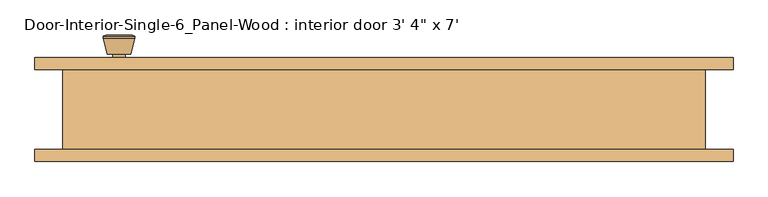
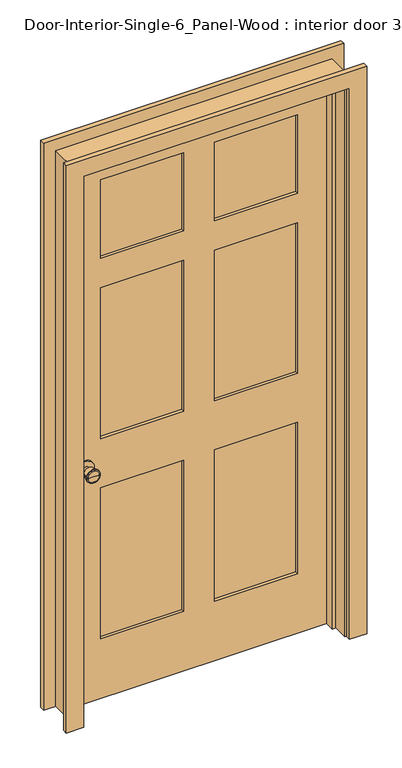
"""IFC4 building model written with IfcOpenShell, lengths in millimetres: door geometry."""

from ifc_helpers import new_model, si_unit, point, frame, frame_2d, origin, place, context, project, spatial, polyline, circle_curve, trimmed, segment, composite_curve, outline, extrude, faceted_brep, source, transform, mapped, element, save
from ifc_brep_helpers import plane_surface, cylinder_surface, revolved_surface, advanced_brep


def door_3d68aebc(model_context):
    return source(origin(), model_context, "Body", "SolidModel", [
        advanced_brep(
        [(-419.1, 19.4, 914.4), (-409.1, 19.4, 914.4), (-429.1, 19.4, 914.4), (-398.6241324, -29.6, 914.4), (-419.1, -29.6, 914.4), (-439.5758676, -29.6, 914.4), (-394.1, -27.7721319, 914.4), (-444.1, -27.7721319, 914.4), (-394.1, -24.3084537, 914.4), (-444.1, -24.3084537, 914.4), (-400.463764, 0.4, 914.4), (-437.736236, 0.4, 914.4), (-409.1, 0.4, 914.4), (-429.1, 0.4, 914.4)],
        [
            (0, 1),
            (1, 2, circle_curve(frame((-419.1, 19.4, 914.4), z_axis=(0.0, 1.0, 0.0), x_axis=(-1.0, 0.0, 0.0)), 10.0)),
            (2, 0),
            (2, 1, circle_curve(frame((-419.1, 19.4, 914.4), z_axis=(0.0, 1.0, 0.0), x_axis=(-1.0, 0.0, 0.0)), 10.0)),
            (3, 4),
            (4, 5),
            (5, 3, circle_curve(frame((-419.1, -29.6, 914.4), z_axis=(0.0, -1.0, 0.0), x_axis=(-1.0, 0.0, 0.0)), 20.4758676)),
            (3, 5, circle_curve(frame((-419.1, -29.6, 914.4), z_axis=(0.0, -1.0, 0.0), x_axis=(-1.0, 0.0, 0.0)), 20.4758676)),
            (6, 3),
            (5, 7),
            (7, 6, circle_curve(frame((-419.1, -27.7721319, 914.4), z_axis=(0.0, -1.0, 0.0), x_axis=(-1.0, 0.0, 0.0)), 25.0)),
            (6, 7, circle_curve(frame((-419.1, -27.7721319, 914.4), z_axis=(0.0, -1.0, 0.0), x_axis=(-1.0, 0.0, 0.0)), 25.0)),
            (8, 6),
            (7, 9),
            (9, 8, circle_curve(frame((-419.1, -24.3084537, 914.4), z_axis=(0.0, -1.0, 0.0), x_axis=(-1.0, 0.0, 0.0)), 25.0)),
            (8, 9, circle_curve(frame((-419.1, -24.3084537, 914.4), z_axis=(0.0, -1.0, 0.0), x_axis=(-1.0, 0.0, 0.0)), 25.0)),
            (10, 8),
            (9, 11),
            (11, 10, circle_curve(frame((-419.1, 0.4, 914.4), z_axis=(0.0, -1.0, 0.0), x_axis=(-1.0, 0.0, 0.0)), 18.636236)),
            (10, 11, circle_curve(frame((-419.1, 0.4, 914.4), z_axis=(0.0, -1.0, 0.0), x_axis=(-1.0, 0.0, 0.0)), 18.636236)),
            (12, 10),
            (11, 13),
            (13, 12, circle_curve(frame((-419.1, 0.4, 914.4), z_axis=(0.0, -1.0, 0.0), x_axis=(-1.0, 0.0, 0.0)), 10.0)),
            (12, 13, circle_curve(frame((-419.1, 0.4, 914.4), z_axis=(0.0, -1.0, 0.0), x_axis=(-1.0, 0.0, 0.0)), 10.0)),
            (1, 12),
            (13, 2),
        ],
        [
            plane_surface(frame((-419.1, 19.4, 914.4), z_axis=(0.0, 1.0, 0.0), x_axis=(-1.0, 0.0, 0.0))),
            plane_surface(frame((-419.1, -29.6, 914.4), z_axis=(0.0, -1.0, 0.0), x_axis=(-1.0, 0.0, 0.0))),
            revolved_surface(polyline([(-439.5758676, -29.6, 914.4), (-444.1, -27.7721319, 914.4)]), (-419.1, 19.4, 914.4), (0.0, 1.0, 0.0)),
            cylinder_surface(frame((-419.1, 19.4, 914.4), z_axis=(0.0, 1.0, 0.0), x_axis=(-1.0, 0.0, 0.0)), 25.0),
            revolved_surface(polyline([(-444.1, -24.3084537, 914.4), (-437.736236, 0.4, 914.4)]), (-419.1, 19.4, 914.4), (0.0, 1.0, 0.0)),
            plane_surface(frame((-419.1, 0.4, 914.4), z_axis=(0.0, 1.0, 0.0), x_axis=(-1.0, 0.0, 0.0))),
            cylinder_surface(frame((-419.1, 19.4, 914.4), z_axis=(0.0, 1.0, 0.0), x_axis=(-1.0, 0.0, 0.0)), 10.0),
        ],
        [
            (0, [[1, 2, 3]]),
            (0, [[-3, 4, -1]]),
            (1, [[5, 6, 7]]),
            (1, [[-6, -5, 8]]),
            (2, [[9, -7, 10, 11]]),
            (2, [[-10, -8, -9, 12]]),
            (3, [[13, -11, 14, 15]]),
            (3, [[-14, -12, -13, 16]]),
            (4, [[17, -15, 18, 19]]),
            (4, [[-18, -16, -17, 20]]),
            (5, [[21, -19, 22, 23]]),
            (5, [[-22, -20, -21, 24]]),
            (6, [[25, -23, 26, -2]]),
            (6, [[-26, -24, -25, -4]]),
        ],
    ),
        extrude(outline(composite_curve([segment(trimmed(circle_curve(frame_2d((914.4, -419.1)), 30.0), [point((914.4, -449.1))], [point((914.4, -389.1))], False, "CARTESIAN"), True, "CONTINUOUS"), segment(trimmed(circle_curve(frame_2d((914.4, -419.1)), 30.0), [point((914.4, -389.1))], [point((914.4, -449.1))], False, "CARTESIAN"), True, "CONTINUOUS")], self_intersect=False)), frame((0.0, 19.4, 0.0), z_axis=(0.0, 1.0, 0.0), x_axis=(0.0, 0.0, 1.0)), (0.0, 0.0, 1.0), 6.0),
        advanced_brep(
        [(-419.1, 66.325, 914.4), (-429.1, 66.325, 914.4), (-409.1, 66.325, 914.4), (-398.6241324, 115.325, 914.4), (-439.5758676, 115.325, 914.4), (-419.1, 115.325, 914.4), (-394.1, 113.4971319, 914.4), (-444.1, 113.4971319, 914.4), (-394.1, 110.0334537, 914.4), (-444.1, 110.0334537, 914.4), (-400.463764, 85.325, 914.4), (-437.736236, 85.325, 914.4), (-409.1, 85.325, 914.4), (-429.1, 85.325, 914.4)],
        [
            (0, 1),
            (1, 2, circle_curve(frame((-419.1, 66.325, 914.4), z_axis=(0.0, -1.0, 0.0), x_axis=(-1.0, 0.0, 0.0)), 10.0)),
            (2, 0),
            (2, 1, circle_curve(frame((-419.1, 66.325, 914.4), z_axis=(0.0, -1.0, 0.0), x_axis=(-1.0, 0.0, 0.0)), 10.0)),
            (3, 4, circle_curve(frame((-419.1, 115.325, 914.4), z_axis=(0.0, 1.0, 0.0), x_axis=(-1.0, 0.0, 0.0)), 20.4758676)),
            (4, 5),
            (5, 3),
            (4, 3, circle_curve(frame((-419.1, 115.325, 914.4), z_axis=(0.0, 1.0, 0.0), x_axis=(-1.0, 0.0, 0.0)), 20.4758676)),
            (6, 7, circle_curve(frame((-419.1, 113.4971319, 914.4), z_axis=(0.0, 1.0, 0.0), x_axis=(-1.0, 0.0, 0.0)), 25.0)),
            (7, 4),
            (3, 6),
            (7, 6, circle_curve(frame((-419.1, 113.4971319, 914.4), z_axis=(0.0, 1.0, 0.0), x_axis=(-1.0, 0.0, 0.0)), 25.0)),
            (8, 9, circle_curve(frame((-419.1, 110.0334537, 914.4), z_axis=(0.0, 1.0, 0.0), x_axis=(-1.0, 0.0, 0.0)), 25.0)),
            (9, 7),
            (6, 8),
            (9, 8, circle_curve(frame((-419.1, 110.0334537, 914.4), z_axis=(0.0, 1.0, 0.0), x_axis=(-1.0, 0.0, 0.0)), 25.0)),
            (10, 11, circle_curve(frame((-419.1, 85.325, 914.4), z_axis=(0.0, 1.0, 0.0), x_axis=(-1.0, 0.0, 0.0)), 18.636236)),
            (11, 9),
            (8, 10),
            (11, 10, circle_curve(frame((-419.1, 85.325, 914.4), z_axis=(0.0, 1.0, 0.0), x_axis=(-1.0, 0.0, 0.0)), 18.636236)),
            (12, 13, circle_curve(frame((-419.1, 85.325, 914.4), z_axis=(0.0, 1.0, 0.0), x_axis=(-1.0, 0.0, 0.0)), 10.0)),
            (13, 11),
            (10, 12),
            (13, 12, circle_curve(frame((-419.1, 85.325, 914.4), z_axis=(0.0, 1.0, 0.0), x_axis=(-1.0, 0.0, 0.0)), 10.0)),
            (1, 13),
            (12, 2),
        ],
        [
            plane_surface(frame((-419.1, 66.325, 914.4), z_axis=(0.0, -1.0, 0.0), x_axis=(-1.0, 0.0, 0.0))),
            plane_surface(frame((-419.1, 115.325, 914.4), z_axis=(0.0, 1.0, 0.0), x_axis=(-1.0, 0.0, 0.0))),
            revolved_surface(polyline([(-439.5758676, 115.325, 914.4), (-444.1, 113.4971319, 914.4)]), (-419.1, 66.325, 914.4), (0.0, -1.0, 0.0)),
            cylinder_surface(frame((-419.1, 66.325, 914.4), z_axis=(0.0, -1.0, 0.0), x_axis=(-1.0, 0.0, 0.0)), 25.0),
            revolved_surface(polyline([(-444.1, 110.0334537, 914.4), (-437.736236, 85.325, 914.4)]), (-419.1, 66.325, 914.4), (0.0, -1.0, 0.0)),
            plane_surface(frame((-419.1, 85.325, 914.4), z_axis=(0.0, -1.0, 0.0), x_axis=(-1.0, 0.0, 0.0))),
            cylinder_surface(frame((-419.1, 66.325, 914.4), z_axis=(0.0, -1.0, 0.0), x_axis=(-1.0, 0.0, 0.0)), 10.0),
        ],
        [
            (0, [[1, 2, 3]]),
            (0, [[-3, 4, -1]]),
            (1, [[5, 6, 7]]),
            (1, [[8, -7, -6]]),
            (2, [[9, 10, -5, 11]]),
            (2, [[12, -11, -8, -10]]),
            (3, [[13, 14, -9, 15]]),
            (3, [[16, -15, -12, -14]]),
            (4, [[17, 18, -13, 19]]),
            (4, [[20, -19, -16, -18]]),
            (5, [[21, 22, -17, 23]]),
            (5, [[24, -23, -20, -22]]),
            (6, [[-2, 25, -21, 26]]),
            (6, [[-4, -26, -24, -25]]),
        ],
    ),
        extrude(outline(composite_curve([segment(trimmed(circle_curve(frame_2d((914.4, -419.1)), 30.0), [point((914.4, -449.1))], [point((914.4, -389.1))], False, "CARTESIAN"), True, "CONTINUOUS"), segment(trimmed(circle_curve(frame_2d((914.4, -419.1)), 30.0), [point((914.4, -389.1))], [point((914.4, -449.1))], False, "CARTESIAN"), True, "CONTINUOUS")], self_intersect=False)), frame((0.0, 60.325, 0.0), z_axis=(0.0, 1.0, 0.0), x_axis=(0.0, 0.0, 1.0)), (0.0, 0.0, 1.0), 6.0),
        faceted_brep([(508.0, 60.325, 0.0), (508.0, -66.675, 0.0), (482.6, -66.675, 0.0), (482.6, -9.525, 0.0), (469.9, -9.525, 0.0), (469.9, 25.4, 0.0), (482.6, 25.4, 0.0), (482.6, 60.325, 0.0), (508.0, 60.325, 2159.0), (508.0, -66.675, 2159.0), (-508.0, -66.675, 2159.0), (-508.0, -66.675, 0.0), (-482.6, -66.675, 0.0), (-482.6, -66.675, 2133.6), (482.6, -66.675, 2133.6), (482.6, -9.525, 2133.6), (-482.6, -9.525, 2133.6), (-482.6, -9.525, 0.0), (-469.9, -9.525, 0.0), (-469.9, -9.525, 2120.9), (469.9, -9.525, 2120.9), (469.9, 25.4, 2120.9), (-469.9, 25.4, 2120.9), (-469.9, 25.4, 0.0), (-482.6, 25.4, 0.0), (-482.6, 25.4, 2133.6), (482.6, 25.4, 2133.6), (482.6, 60.325, 2133.6), (-482.6, 60.325, 2133.6), (-482.6, 60.325, 0.0), (-508.0, 60.325, 0.0), (-508.0, 60.325, 2159.0)], [[[0, 1, 2, 3, 4, 5, 6, 7]], [[1, 0, 8, 9]], [[2, 1, 9, 10, 11, 12, 13, 14]], [[3, 2, 14, 15]], [[4, 3, 15, 16, 17, 18, 19, 20]], [[5, 4, 20, 21]], [[6, 5, 21, 22, 23, 24, 25, 26]], [[7, 6, 26, 27]], [[0, 7, 27, 28, 29, 30, 31, 8]], [[9, 8, 31, 10]], [[15, 14, 13, 16]], [[21, 20, 19, 22]], [[27, 26, 25, 28]], [[30, 29, 24, 23, 18, 17, 12, 11]], [[10, 31, 30, 11]], [[16, 13, 12, 17]], [[22, 19, 18, 23]], [[28, 25, 24, 29]]]),
        extrude(outline(polyline([(2133.6, -482.6), (0.0, -482.6), (0.0, 482.6), (2133.6, 482.6), (2133.6, -482.6)]), holes=[polyline([(2014.5375, 57.15), (2014.5375, 361.95), (1709.7375, 361.95), (1709.7375, 57.15), (2014.5375, 57.15)]), polyline([(1595.4375, 361.95), (1009.65, 361.95), (1009.65, 57.15), (1595.4375, 57.15), (1595.4375, 361.95)]), polyline([(1009.65, -57.15), (1009.65, -361.95), (1595.4375, -361.95), (1595.4375, -57.15), (1009.65, -57.15)]), polyline([(1709.7375, -361.95), (2014.5375, -361.95), (2014.5375, -57.15), (1709.7375, -57.15), (1709.7375, -361.95)]), polyline([(819.15, 57.15), (819.15, 361.95), (231.775, 361.95), (231.775, 57.15), (819.15, 57.15)]), polyline([(231.775, -57.15), (231.775, -361.95), (819.15, -361.95), (819.15, -57.15), (231.775, -57.15)])]), frame((0.0, 25.4, 0.0), z_axis=(0.0, 1.0, 0.0), x_axis=(0.0, 0.0, 1.0)), (0.0, 0.0, 1.0), 34.925),
        extrude(outline(polyline([(361.95, 37.0416667), (57.15, 37.0416667), (57.15, 48.6833333), (361.95, 48.6833333), (361.95, 37.0416667)])), frame((0.0, 0.0, 1709.7375), z_axis=(0.0, 0.0, 1.0), x_axis=(1.0, 0.0, 0.0)), (0.0, 0.0, 1.0), 304.8),
        extrude(outline(polyline([(361.95, 37.0416667), (57.15, 37.0416667), (57.15, 48.6833333), (361.95, 48.6833333), (361.95, 37.0416667)])), frame((0.0, 0.0, 1009.65), z_axis=(0.0, 0.0, 1.0), x_axis=(1.0, 0.0, 0.0)), (0.0, 0.0, 1.0), 585.7875),
        extrude(outline(polyline([(-57.15, 37.0416667), (-361.95, 37.0416667), (-361.95, 48.6833333), (-57.15, 48.6833333), (-57.15, 37.0416667)])), frame((0.0, 0.0, 1009.65), z_axis=(0.0, 0.0, 1.0), x_axis=(1.0, 0.0, 0.0)), (0.0, 0.0, 1.0), 585.7875),
        extrude(outline(polyline([(-57.15, 37.0416667), (-361.95, 37.0416667), (-361.95, 48.6833333), (-57.15, 48.6833333), (-57.15, 37.0416667)])), frame((0.0, 0.0, 1709.7375), z_axis=(0.0, 0.0, 1.0), x_axis=(1.0, 0.0, 0.0)), (0.0, 0.0, 1.0), 304.8),
        extrude(outline(polyline([(361.95, 37.0416667), (57.15, 37.0416667), (57.15, 48.6833333), (361.95, 48.6833333), (361.95, 37.0416667)])), frame((0.0, 0.0, 231.775), z_axis=(0.0, 0.0, 1.0), x_axis=(1.0, 0.0, 0.0)), (0.0, 0.0, 1.0), 587.375),
        extrude(outline(polyline([(-57.15, 37.0416667), (-361.95, 37.0416667), (-361.95, 48.6833333), (-57.15, 48.6833333), (-57.15, 37.0416667)])), frame((0.0, 0.0, 231.775), z_axis=(0.0, 0.0, 1.0), x_axis=(1.0, 0.0, 0.0)), (0.0, 0.0, 1.0), 587.375),
        extrude(outline(polyline([(0.0, 488.95), (0.0, 552.45), (2203.45, 552.45), (2203.45, -552.45), (0.0, -552.45), (0.0, -488.95), (2139.95, -488.95), (2139.95, 488.95), (0.0, 488.95)])), frame((0.0, 60.325, 0.0), z_axis=(0.0, 1.0, 0.0), x_axis=(0.0, 0.0, 1.0)), (0.0, 0.0, 1.0), 19.05),
        extrude(outline(polyline([(0.0, 488.95), (0.0, 552.45), (2203.45, 552.45), (2203.45, -552.45), (0.0, -552.45), (0.0, -488.95), (2139.95, -488.95), (2139.95, 488.95), (0.0, 488.95)])), frame((0.0, -85.725, 0.0), z_axis=(0.0, 1.0, 0.0), x_axis=(0.0, 0.0, 1.0)), (0.0, 0.0, 1.0), 19.05),
    ])


if __name__ == "__main__":
    model = new_model("IFC4")
    model_context = context("Model", 3, world=origin())
    ifc_project = project(units=[si_unit("LENGTHUNIT", "METRE", prefix="MILLI")], contexts=[model_context])
    site = spatial("IfcSite", under=ifc_project)
    building = spatial("IfcBuilding", under=site)
    placement = place(None, origin())
    door_shape = door_3d68aebc(model_context)
    element("IfcDoor", 1, ObjectType="Door-Interior-Single-6_Panel-Wood : interior door 3' 4\" x 7'", at=placement, inside=building, context=model_context, shape_type="MappedRepresentation", body=[
        mapped(door_shape, transform((0.0, 0.0, 0.0), x_axis=(1.0, 0.0, 0.0), y_axis=(0.0, 1.0, 0.0), z_axis=(0.0, 0.0, 1.0))),
    ])
    save(model, "model.ifc")

# Revit data of these elements
# Type "Door-Interior-Single-6_Panel-Wood : interior door 3' 4\" x 7'"
#   Type Mark = "11"
#   Assembly Code = "C1020300"
#   Analytic Construction = "Wooden"
#   Top Rail = 0' - 4 11/16"
#   Top Panel = 1' - 0"
#   Thickness = 0' - 1 3/8"
#   Thermal Resistance (R) = 2.5876 (h·ft²·°F)/BTU
#   Swing Angle [instance default] = 90.00°
#   Stiles = 0' - 4 3/4"
#   Rough Width = 3' - 4"
#   Rough Height = 7' - 1"
#   Mullion = 0' - 4 1/2"
#   Lock Rail = 0' - 7 1/2"
#   Intermediate Rail = 0' - 4 1/2"
#   Height = 7' - 0"
#   Width = 3' - 2"
#   Heat Transfer Coefficient (U) = 0.3865 BTU/(h·ft²·°F)
#   Bottom Rail = 0' - 9 1/8"
#   Trim Material = Cherry
#   Panel Material = Cherry
#   Frame Material = Cherry
#   Door Handle Material = Aluminum
#   Visual Light Transmittance = 0
#   Solar Heat Gain Coefficient = 0
#   Wall Closure = (empty or 0)
#   Function = (empty or 0)
# Element 1 (IfcDoor, "Door-Interior-Single-6_Panel-Wood : interior door 3' 4\" x 7'")
#   Materials on its faces: "Cherry", "Aluminum"
# Materials
#   "Cherry": class "Wood", colour RGB 226 177 128, transparency 0, Description = "Prunus Serotina", Cost = 0
#   "Aluminum": class "Metal", colour RGB 247 247 247, transparency 0, Description = "Aluminum 6061", Cost = 0
